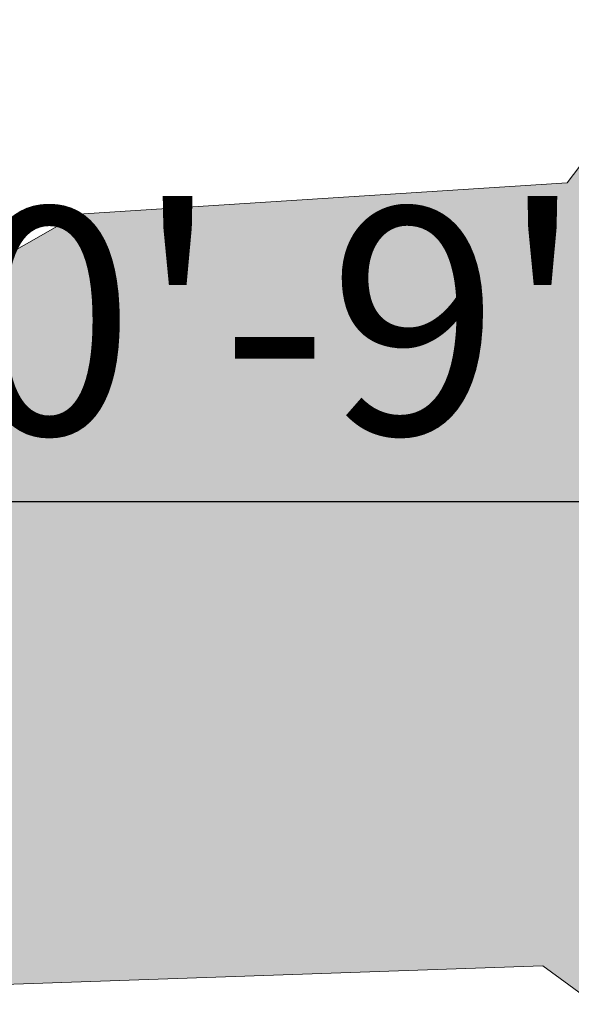
# Model space of a CAD drawing. Units: inches. Extents: x 2091 to 2899, y 967 to 2217.
# Tile 252 of 256: x 2221.88 to 2231.62, y 1131.25 to 1148.63. Entities that reach past the tile are written whole.
import ezdxf

# ---------------------------------------------------------------- set-up
doc = ezdxf.new("R2010")
doc.units = ezdxf.units.IN
doc.layers.add('A-ANNO-DIMS', color=2, linetype='Continuous', lineweight=18)
doc.layers.add('L-PLNT-TREE', color=94, linetype='Continuous', lineweight=13)
doc.layers.add('A-WALL-PATT', color=141, linetype='Continuous', lineweight=13, true_color=0xadddf7)
doc.layers.add('L-PLNT-PATT', color=114, linetype='Continuous', lineweight=13, true_color=0x139b48)
doc.styles.get("Standard").update_dxf_attribs({"font": 'arial.ttf'})
doc.dimstyles.new('ISO-25', dxfattribs={"dimtxt": 4, "dimasz": 4, "dimexe": 1.25, "dimexo": 0.625, "dimtad": 1, "dimdec": 0, "dimlunit": 3, "dimtxsty": 'Standard', "dimcen": 2.5, "dimadec": 0, "dimazin": 0, "dimtfac": 1, "dimtdec": 0, "dimtmove": 0, "dimatfit": 3, "dimfxl": 1, "dimarcsym": 0})

# ---------------------------------------------------------------- blocks, each defined once
blk = doc.blocks.new('*U25')
blk.add_lwpolyline([(-1139.42368, 1783.79628), (-1216.11644, 1685.47796), (-1117.5111, 1601.2033), (-1051.7759, 1643.3419), (-1126.09884, 1521.20092), (-1072.10606, 1527.49758), (-1079.90386, 1416.93646), (-1259.93906, 1179.83508), (-1479.05978, 1165.78888), (-1577.66258, 1109.60662), (-1742.00312, 927.01364), (-1676.26538, 814.64658), (-1270.89408, 828.69278), (-1194.20386, 772.51052), (-1007.95074, 856.78518), (-876.4778, 575.87134), (-821.70016, 575.87134), (-569.71184, 884.87504)])
blk = doc.blocks.new('*D37')
at = {"layer": 'A-ANNO-DIMS', "color": 0, "lineweight": -2, "transparency": 16777216}
for p, q in [((2203.116, 1151.622), (2203.116, 1138.874)), ((2212.276, 1151.622), (2212.276, 1138.874)), ((2199.116, 1140.124), (2195.116, 1140.124)), ((2203.116, 1140.124), (2212.276, 1140.124)), ((2216.276, 1140.124), (2245.908, 1140.124))]:
    blk.add_line(p, q, dxfattribs=at)
at = {"layer": 'A-ANNO-DIMS', "color": 0, "transparency": 16777216}
for points in [[(2199.116, 1140.79), (2199.116, 1139.457), (2203.116, 1140.124)], [(2216.276, 1140.79), (2216.276, 1139.457), (2212.276, 1140.124)]]:
    blk.add_solid(points, dxfattribs=at)
at = {"layer": 'Defpoints', "color": 0, "transparency": 16777216}
for p in [(2203.116, 1152.247), (2212.276, 1152.247), (2212.276, 1140.124)]:
    blk.add_point(p, dxfattribs=at)
at = {"layer": 'A-ANNO-DIMS', "color": 0, "transparency": 16777216, "insert": (2233.092, 1142.791), "char_height": 4, "attachment_point": 5}
blk.add_mtext('0\'-9" TYP.', dxfattribs=at)
blk = doc.blocks.new('*D71')
at = {"layer": 'A-ANNO-DIMS', "color": 0, "lineweight": -2, "transparency": 16777216}
for p, q in [((2212.144, 1351.294), (2212.144, 969.464)), ((2452.144, 1351.294), (2452.144, 969.464)), ((2216.144, 970.714), (2448.144, 970.714))]:
    blk.add_line(p, q, dxfattribs=at)
at = {"layer": 'A-ANNO-DIMS', "color": 0, "transparency": 16777216}
for points in [[(2216.144, 971.381), (2216.144, 970.048), (2212.144, 970.714)], [(2448.144, 971.381), (2448.144, 970.048), (2452.144, 970.714)]]:
    blk.add_solid(points, dxfattribs=at)
at = {"layer": 'Defpoints', "color": 0, "transparency": 16777216}
for p in [(2212.144, 1351.919), (2452.144, 1351.919), (2452.144, 970.714)]:
    blk.add_point(p, dxfattribs=at)
at = {"layer": 'A-ANNO-DIMS', "color": 0, "transparency": 16777216, "insert": (2332.144, 973.382), "char_height": 4, "attachment_point": 5}
blk.add_mtext('20\'-0"', dxfattribs=at)

msp = doc.modelspace()

# ---------------------------------------------------------------- hatches: boundary and pattern name
at = {"layer": 'A-WALL-PATT'}
h = msp.add_hatch(color=256, dxfattribs=at)
h.dxf.hatch_style = 1
h.paths.add_polyline_path([(2803.144, 2050.919), (2203.144, 2050.919), (2203.144, 1090.919), (2803.144, 1090.919)])
h.paths.add_polyline_path([(2635.799, 1147.54), (2674.524, 1147.54, 0.376086), (2678.53, 1152.88), (2678.53, 1159.556, 0.333335), (2674.524, 1163.562), (2674.524, 1163.562), (2674.524, 1192.934), (2635.806, 1192.934), (2597.088, 1192.934), (2597.088, 1163.562, 0.333335), (2593.082, 1159.556), (2593.082, 1152.88, 0.376086), (2597.088, 1147.54)], flags=0)
h.paths.add_polyline_path([(2436.01, 1278.241, 0.000483), (2435.953, 1278.215, -0.001328), (2435.936, 1278.112, -0.001711), (2436.116, 1278.041, 0.002185)], flags=0)
h.paths.add_polyline_path([(2794.144, 1143.419), (2794.144, 1347.419), (2543.37, 1347.419), (2543.37, 1351.919), (2794.144, 1351.919), (2794.144, 1392.714), (2793.947, 1392.714), (2793.947, 1473.537), (2794.144, 1473.537), (2794.144, 1531.919), (2650.144, 1531.919), (2650.144, 1536.419), (2794.144, 1536.419), (2794.144, 1692.419), (2609.376, 1692.419), (2609.376, 1644.419), (2604.876, 1644.419), (2604.876, 1744.919), (2609.376, 1744.919), (2609.376, 1696.919), (2794.144, 1696.919), (2794.144, 1780.919), (2609.644, 1780.919), (2493.876, 1780.919), (2493.876, 1785.419), (2609.644, 1785.419), (2794.144, 1785.419), (2794.144, 1847.939), (2793.951, 1847.939), (2793.951, 1928.762), (2794.144, 1928.762), (2794.144, 1941.419), (2614.144, 1941.419), (2614.144, 1821.419), (2609.644, 1821.419), (2609.644, 1941.419), (2392.144, 1941.419), (2392.144, 1819.919), (2387.644, 1819.919), (2387.644, 1941.419), (2212.144, 1941.419), (2212.144, 1783.919), (2392.144, 1783.919), (2392.144, 1780.919), (2212.144, 1780.919), (2212.144, 1629.419), (2387.644, 1629.419), (2387.644, 1744.919), (2392.144, 1744.919), (2392.144, 1627.919), (2317.144, 1627.919), (2317.144, 1551.419), (2317.144, 1536.419), (2459.384, 1536.419), (2459.384, 1602.396), (2463.884, 1602.396), (2463.884, 1531.919), (2456.644, 1531.919), (2456.644, 1529.919), (2452.144, 1529.919), (2452.144, 1531.919), (2312.644, 1531.919), (2312.644, 1551.419), (2306.144, 1551.419), (2306.144, 1555.919), (2308.144, 1555.919), (2308.144, 1551.419), (2312.644, 1551.419), (2312.644, 1627.919), (2212.144, 1627.919), (2212.144, 1555.919), (2270.144, 1555.919), (2270.144, 1551.419), (2212.144, 1551.419), (2212.144, 1351.919), (2272.144, 1351.919), (2272.144, 1347.419), (2212.144, 1347.419), (2212.144, 1275.419), (2308.144, 1275.419), (2308.144, 1351.919), (2452.144, 1351.919), (2452.144, 1493.919), (2456.644, 1493.919), (2456.644, 1347.419), (2312.644, 1347.419), (2312.644, 1270.919), (2212.144, 1270.919), (2212.144, 1099.919), (2281.238, 1099.919), (2282.871, 1110.914), (2282.008, 1116.997), (2278.558, 1121.42), (2268.206, 1128.056), (2272.088, 1128.056), (2273.813, 1131.927), (2279.42, 1134.692), (2285.028, 1135.245), (2287.616, 1137.457), (2288.047, 1138.01), (2289.341, 1140.775), (2291.067, 1139.669), (2292.361, 1135.245), (2295.38, 1136.904), (2296.243, 1135.798), (2297.105, 1133.033), (2300.125, 1138.01), (2303.144, 1138.01), (2304.438, 1135.798), (2303.144, 1133.586), (2306.595, 1134.692), (2307.889, 1133.033), (2310.908, 1135.245), (2313.927, 1134.139), (2315.627, 1132.427), (2308.32, 1117.55), (2290.204, 1109.808), (2288.91, 1103.172), (2289.272, 1099.919), (2434.918, 1099.919), (2431.593, 1124.788), (2429.93, 1169.553), (2430.927, 1240.52), (2435.659, 1238.186), (2437.135, 1196.554), (2438.798, 1143.973), (2442.678, 1111.998), (2446.558, 1099.919), (2794.144, 1099.919), (2794.144, 1138.919), (2548.032, 1138.919), (2548.032, 1143.419), (2548.032, 1148.819), (2546.668, 1148.032), (2528.686, 1179.179, 0.256256), (2512.032, 1148.819), (2512.032, 1143.419), (2512.032, 1138.919), (2507.532, 1138.919), (2507.532, 1143.419), (2507.532, 1148.819, 0.256256), (2490.879, 1179.179), (2472.896, 1148.032), (2471.532, 1148.819), (2471.532, 1143.419), (2467.032, 1143.419), (2467.032, 1269.946, 0.039061), (2460.91, 1273.58), (2467.032, 1273.58), (2467.032, 1286.325, 0.014511), (2465.216, 1286.762), (2467.032, 1287.053), (2467.032, 1323.419), (2471.532, 1323.419), (2471.532, 1148.819), (2489.532, 1179.996), (2490.896, 1179.208), (2490.879, 1179.179, -0.256256), (2507.532, 1148.819), (2507.532, 1143.419), (2512.032, 1143.419), (2512.032, 1148.819, -0.256256), (2528.686, 1179.179), (2528.668, 1179.208), (2530.032, 1179.996), (2548.032, 1148.819), (2548.032, 1143.419)], flags=16)
h.paths.add_polyline_path([(2607.769, 1200.945), (2607.769, 1265.031), (2597.088, 1281.052), (2619.785, 1281.052), (2627.795, 1337.127), (2635.799, 1337.127), (2643.817, 1337.127), (2651.827, 1281.052), (2674.524, 1281.052), (2663.843, 1265.031), (2663.843, 1200.945), (2635.806, 1200.945)], flags=0)
edge = h.paths.add_edge_path(flags=0)
edge.add_ellipse((13303.896, 1272.999), major_axis=(-10595.313, 0), ratio=0.84230387, start_angle=0.6282372, end_angle=0.6465541, ccw=False)
edge.add_ellipse((2711.7, 1156.853), major_axis=(2.22, 0), ratio=0.842304, start_angle=111.5352, end_angle=180.6282, ccw=False)
edge.add_ellipse((13303.156, 1272.999), major_axis=(-10593.026, 0), ratio=0.84230387, start_angle=0.5282715, end_angle=0.6465541, ccw=False)
edge.add_line((2710.765, 1175.333), (2710.13, 1175.333))
edge.add_ellipse((2710.13, 1176.58), major_axis=(1.48, 0), ratio=0.842304, start_angle=180, end_angle=270, ccw=False)
edge.add_line((2708.65, 1176.58), (2708.65, 1200.783))
edge.add_ellipse((2710.13, 1200.783), major_axis=(1.48, 0), ratio=0.842304, start_angle=90, end_angle=180, ccw=False)
edge.add_line((2710.13, 1202.029), (2710.465, 1202.029))
edge.add_ellipse((13303.156, 1272.999), major_axis=(-10593.026, 0), ratio=0.84230387, start_angle=-0.0902291, end_angle=0.3838668, ccw=False)
edge.add_ellipse((2710.13, 1290.927), major_axis=(-1.48, 0), ratio=0.842304, start_angle=0, end_angle=90, ccw=False)
edge.add_line((2708.65, 1290.927), (2708.65, 1315.13))
edge.add_ellipse((2710.13, 1315.13), major_axis=(-1.48, 0), ratio=0.842304, start_angle=-90, end_angle=0, ccw=False)
edge.add_line((2710.13, 1316.377), (2710.706, 1316.377))
edge.add_ellipse((3238.402, 1296.29), major_axis=(528.234, 0), ratio=0.8423039, start_angle=176.34957, end_angle=177.82005, ccw=False)
edge.add_ellipse((2775.063, 1071.451), major_axis=(313.308, 0), ratio=0.8423039, start_angle=102.12597, end_angle=103.78053, ccw=False)
edge.add_ellipse((2775.063, 1078.306), major_axis=(-305.303, 0), ratio=0.8423039, start_angle=-79.79046, end_angle=-77.55537, ccw=False)
edge.add_ellipse((2695.142, 1541.975), major_axis=(-250.96, 0), ratio=0.8423039, start_angle=99.25657, end_angle=102.55493)
edge.add_line((2741.41, 1334.214), (2747.133, 1337.378))
edge.add_ellipse((2747.539, 1336.857), major_axis=(-0.74, 0), ratio=0.842304, start_angle=270, end_angle=307.9331, ccw=False)
edge.add_ellipse((2747.539, 1336.857), major_axis=(-0.74, 0), ratio=0.842304, start_angle=232.0669, end_angle=270, ccw=False)
edge.add_line((2747.945, 1337.378), (2753.667, 1334.214))
edge.add_ellipse((2799.935, 1541.975), major_axis=(250.96, 0), ratio=0.8423039, start_angle=257.44507, end_angle=260.74343)
edge.add_ellipse((2720.014, 1078.306), major_axis=(305.303, 0), ratio=0.8423039, start_angle=77.55537, end_angle=79.79046, ccw=False)
edge.add_ellipse((2720.014, 1071.451), major_axis=(-313.308, 0), ratio=0.8423039, start_angle=256.21947, end_angle=257.87403, ccw=False)
edge.add_ellipse((2256.676, 1296.29), major_axis=(-528.234, 0), ratio=0.8423039, start_angle=182.17995, end_angle=183.65043, ccw=False)
edge.add_line((2784.371, 1316.377), (2784.947, 1316.377))
edge.add_ellipse((2784.947, 1315.13), major_axis=(1.48, 0), ratio=0.842304, start_angle=0, end_angle=90, ccw=False)
edge.add_line((2786.427, 1315.13), (2786.427, 1290.927))
edge.add_ellipse((2784.947, 1290.927), major_axis=(1.48, 0), ratio=0.842304, start_angle=270, end_angle=360, ccw=False)
edge.add_ellipse((-7808.079, 1272.999), major_axis=(10593.026, 0), ratio=0.84230387, start_angle=-0.3838668, end_angle=0.0902291, ccw=False)
edge.add_line((2784.612, 1202.029), (2784.947, 1202.029))
edge.add_ellipse((2784.947, 1200.783), major_axis=(1.48, 0), ratio=0.842304, start_angle=0, end_angle=90, ccw=False)
edge.add_line((2786.427, 1200.783), (2786.427, 1176.58))
edge.add_ellipse((2784.947, 1176.58), major_axis=(-1.48, 0), ratio=0.842304, start_angle=90, end_angle=180, ccw=False)
edge.add_line((2784.947, 1175.333), (2784.313, 1175.333))
edge.add_ellipse((-7808.079, 1272.999), major_axis=(10593.026, 0), ratio=0.84230387, start_angle=-0.6186432, end_angle=-0.5282715, ccw=False)
edge.add_ellipse((2783.377, 1156.853), major_axis=(-2.22, 0), ratio=0.842304, start_angle=179.3718, end_angle=248.4648, ccw=False)
edge.add_ellipse((-7808.819, 1272.999), major_axis=(-10595.313, 0), ratio=0.842303866, start_angle=179.3534459, end_angle=179.3717628, ccw=False)
edge.add_ellipse((2780.297, 1153.501), major_axis=(-5.246, 0), ratio=0.842304, start_angle=90, end_angle=179.3534, ccw=False)
edge.add_line((2780.297, 1149.082), (2714.78, 1149.082))
edge.add_ellipse((2714.78, 1153.501), major_axis=(5.246, 0), ratio=0.842304, start_angle=180.6466, end_angle=270, ccw=False)
edge = h.paths.add_edge_path(flags=0)
edge.add_line((2718.187, 1151.008), (2718.187, 1170.472))
edge.add_ellipse((2721.147, 1170.472), major_axis=(-2.96, 0), ratio=0.842304, start_angle=-90, end_angle=0, ccw=False)
edge.add_line((2721.147, 1172.965), (2773.93, 1172.965))
edge.add_ellipse((2773.93, 1170.472), major_axis=(-2.96, 0), ratio=0.842304, start_angle=180, end_angle=270, ccw=False)
edge.add_line((2776.89, 1170.472), (2776.89, 1151.008))
edge.add_line((2776.89, 1151.008), (2718.187, 1151.008))
edge = h.paths.add_edge_path(flags=0)
edge.add_line((2718.187, 1180.234), (2718.187, 1199.058))
edge.add_ellipse((2747.539, 1320.399), major_axis=(147.018, 0), ratio=0.8423039, start_angle=256.40187, end_angle=283.59813)
edge.add_line((2776.89, 1199.058), (2776.89, 1180.234))
edge.add_ellipse((2747.539, 1301.575), major_axis=(147.018, 0), ratio=0.8423039, start_angle=256.40187, end_angle=283.59813, ccw=False)
edge = h.paths.add_edge_path(flags=0)
edge.add_ellipse((13303.156, 1272.999), major_axis=(-10591.546, 0), ratio=0.84230387, start_angle=0.0555943, end_angle=0.3777642, ccw=False)
edge.add_line((2711.617, 1262.722), (2715.667, 1249.495))
edge.add_ellipse((6413.892, 1241.692), major_axis=(-3698.236, 0), ratio=0.84230387, start_angle=-0.120897, end_angle=0.364076)
edge.add_line((2715.761, 1218.192), (2711.934, 1203.167))
edge = h.paths.add_edge_path(flags=0)
edge.add_line((2718.187, 1251.075), (2716.002, 1267.45))
edge.add_ellipse((2742.151, 1202.19), major_axis=(81.773, 0), ratio=0.842304, start_angle=94.27742, end_angle=111.83495, ccw=False)
edge.add_line((2737.01, 1270.931), (2758.067, 1270.931))
edge.add_ellipse((2752.926, 1202.19), major_axis=(81.773, 0), ratio=0.842304, start_angle=68.16505, end_angle=85.72258, ccw=False)
edge.add_line((2779.075, 1267.45), (2776.89, 1251.075))
edge.add_ellipse((2750.338, 1187.885), major_axis=(79.58, 0), ratio=0.842304, start_angle=67.20809, end_angle=85.12993)
edge.add_line((2756.035, 1254.744), (2739.043, 1254.744))
edge.add_ellipse((2744.739, 1187.885), major_axis=(79.58, 0), ratio=0.842304, start_angle=94.87007, end_angle=112.79191)
edge = h.paths.add_edge_path(flags=0)
edge.add_line((2783.143, 1203.167), (2779.316, 1218.192))
edge.add_ellipse((-918.815, 1241.692), major_axis=(3698.236, 0), ratio=0.84230387, start_angle=-0.364076, end_angle=0.120897)
edge.add_line((2779.41, 1249.495), (2783.46, 1262.722))
edge.add_ellipse((-7808.079, 1272.999), major_axis=(-10591.546, 0), ratio=0.84230387, start_angle=179.6222358, end_angle=179.9444057, ccw=False)
edge = h.paths.add_edge_path(flags=0)
edge.add_ellipse((2734.201, 1286.69), major_axis=(-0.357, 6.34), ratio=0.603834, start_angle=89.002, end_angle=253.6574, ccw=False)
edge.add_line((2730.369, 1286.542), (2730.369, 1301.352))
edge.add_line((2730.369, 1301.352), (2735.913, 1305.215))
edge.add_ellipse((2736.385, 1304.735), major_axis=(0.74, 0), ratio=0.842304, start_angle=90, end_angle=134.4802, ccw=False)
edge.add_line((2736.385, 1305.358), (2738.033, 1305.358))
edge.add_line((2738.033, 1305.358), (2738.033, 1307.708))
edge.add_ellipse((2794.202, 1307.708), major_axis=(56.169, 0), ratio=0.842304, start_angle=150.5614, end_angle=180, ccw=False)
edge.add_ellipse((2700.876, 1307.708), major_axis=(-56.169, 0), ratio=0.842304, start_angle=180, end_angle=209.4386, ccw=False)
edge.add_line((2757.044, 1307.708), (2757.044, 1305.358))
edge.add_line((2757.044, 1305.358), (2758.692, 1305.358))
edge.add_ellipse((2758.692, 1304.735), major_axis=(-0.74, 0), ratio=0.842304, start_angle=225.5198, end_angle=270, ccw=False)
edge.add_line((2759.164, 1305.215), (2764.708, 1301.352))
edge.add_line((2764.708, 1301.352), (2764.708, 1286.542))
edge.add_ellipse((2760.876, 1286.69), major_axis=(0.357, 6.34), ratio=0.603834, start_angle=106.3426, end_angle=270.998, ccw=False)
edge.add_line((2757.044, 1285.797), (2757.044, 1307.708))
edge.add_ellipse((2700.876, 1307.708), major_axis=(-56.169, 0), ratio=0.842304, start_angle=180, end_angle=209.4386)
edge.add_ellipse((2794.202, 1307.708), major_axis=(56.169, 0), ratio=0.842304, start_angle=150.5614, end_angle=180)
edge.add_line((2738.033, 1307.708), (2738.033, 1285.797))
h.paths.add_polyline_path([(2417.812, 1104.45), (2413.492, 1102.53), (2410.612, 1103.97), (2409.172, 1106.37), (2407.252, 1107.33), (2406.292, 1109.73), (2405.332, 1114.05), (2405.332, 1117.89), (2406.292, 1120.13), (2407.252, 1119.81), (2408.848, 1118.328), (2410.174, 1119.424), (2410.211, 1120.406), (2411.041, 1121.419), (2410.699, 1119.859), (2410.174, 1119.424), (2410.088, 1117.176), (2411.133, 1116.206), (2413.972, 1119.33), (2416.852, 1120.77), (2416.87, 1120.799), (2417.035, 1119.405), (2417.896, 1118.143), (2418.292, 1118.37), (2419.544, 1120.039), (2419.361, 1118.387), (2419.032, 1119.356), (2418.399, 1118.512), (2419.252, 1114.53), (2418.794, 1107.199)], flags=0)
h.paths.add_polyline_path([(2508.87, 1347.419), (2508.37, 1347.419), (2508.37, 1351.919), (2508.87, 1351.919)], flags=0)
h.paths.add_polyline_path([(2473.37, 1347.419), (2472.37, 1347.419), (2467.87, 1347.419), (2467.87, 1455.419), (2472.37, 1455.419), (2472.37, 1352.419), (2473.37, 1352.419)], flags=0)
h.paths.add_polyline_path([(2352.106, 1217.446), (2349.226, 1218.886), (2347.786, 1221.286), (2345.866, 1222.246), (2344.906, 1224.646), (2343.946, 1228.966), (2343.946, 1232.806), (2344.906, 1235.046), (2345.866, 1234.726), (2347.462, 1233.244), (2348.788, 1234.341), (2348.825, 1235.322), (2349.655, 1236.336), (2349.313, 1234.775), (2348.788, 1234.341), (2348.702, 1232.093), (2349.747, 1231.123), (2352.586, 1234.246), (2355.466, 1235.686), (2355.484, 1235.715), (2355.649, 1234.322), (2356.51, 1233.06), (2356.906, 1233.286), (2358.158, 1234.956), (2357.975, 1233.304), (2357.646, 1234.273), (2357.013, 1233.428), (2357.866, 1229.446), (2357.408, 1222.115), (2356.426, 1219.366)], flags=0)
h.paths.add_polyline_path([(2348.297, 1112.224), (2347.014, 1112.31), (2345.53, 1114.127), (2345.732, 1115.858), (2346.812, 1116.982), (2346.812, 1114.646), (2345.867, 1114.214), (2346.88, 1114.3)], flags=0)
h.paths.add_polyline_path([(2347.014, 1110.926), (2346.272, 1110.493), (2346.61, 1111.186)], flags=0)
h.paths.add_polyline_path([(2345.867, 1118.194), (2345.53, 1117.329), (2343.708, 1118.021), (2344.383, 1118.626)], flags=0)
h.paths.add_polyline_path([(2346.677, 1109.282), (2346.07, 1108.071), (2345.867, 1110.061)], flags=0)
h.paths.add_polyline_path([(2345.057, 1119.751), (2343.64, 1119.751), (2343.978, 1121.135)], flags=0)
h.paths.add_polyline_path([(2345.26, 1116.55), (2345.125, 1115.858), (2344.922, 1115.685), (2344.72, 1116.377)], flags=0)
h.paths.add_polyline_path([(2345.665, 1112.31), (2345.462, 1111.532), (2344.045, 1111.964), (2344.652, 1112.57)], flags=0)
h.paths.add_polyline_path([(2345.192, 1113.349), (2344.45, 1113.868), (2344.72, 1114.387)], flags=0)
h.paths.add_polyline_path([(2344.652, 1116.809), (2344.18, 1115.685), (2344.652, 1115.339), (2343.91, 1114.906), (2343.033, 1115.944), (2343.64, 1116.463)], flags=0)
h.paths.add_polyline_path([(2345.867, 1106.686), (2344.99, 1105.562), (2344.517, 1106.6)], flags=0)
h.paths.add_polyline_path([(2344.855, 1110.061), (2344.517, 1109.282), (2344.113, 1109.715)], flags=0)
h.paths.add_polyline_path([(2344.045, 1113.522), (2343.438, 1113.089), (2342.763, 1113.954)], flags=0)
h.paths.add_polyline_path([(2344.315, 1111.012), (2342.965, 1110.32), (2342.965, 1111.099)], flags=0)
h.paths.add_polyline_path([(2345.125, 1104.697), (2344.585, 1103.745), (2344.45, 1104.264)], flags=0)
h.paths.add_polyline_path([(2342.83, 1121.222), (2341.75, 1120.53), (2340.536, 1121.049), (2340.131, 1121.828), (2340.671, 1122.952), (2341.143, 1121.828), (2341.615, 1122.001)], flags=0)
h.paths.add_polyline_path([(2342.965, 1119.751), (2343.033, 1118.453), (2342.088, 1118.021), (2342.02, 1119.491)], flags=0)
h.paths.add_polyline_path([(2342.695, 1116.896), (2341.953, 1116.636), (2342.02, 1117.329)], flags=0)
h.paths.add_polyline_path([(2343.033, 1112.224), (2342.02, 1111.791), (2341.548, 1112.224), (2342.358, 1113.349)], flags=0)
h.paths.add_polyline_path([(2343.775, 1104.437), (2342.628, 1102.88), (2342.695, 1104.61), (2343.438, 1105.129)], flags=0)
h.paths.add_polyline_path([(2342.02, 1115.079), (2340.806, 1115.512), (2340.941, 1116.377)], flags=0)
h.paths.add_polyline_path([(2341.481, 1120.097), (2341.481, 1119.405), (2341.076, 1119.578), (2341.143, 1120.097)], flags=0)
h.paths.add_polyline_path([(2341.818, 1114.473), (2340.941, 1113.089), (2340.806, 1114.56)], flags=0)
h.paths.add_polyline_path([(2341.143, 1118.54), (2340.941, 1116.982), (2339.051, 1117.675), (2339.051, 1118.626)], flags=0)
h.paths.add_polyline_path([(2342.695, 1101.668), (2341.953, 1101.841), (2342.56, 1102.361)], flags=0)
h.paths.add_polyline_path([(2340.333, 1119.665), (2338.444, 1119.578), (2337.904, 1120.357), (2339.658, 1120.616)], flags=0)
h.paths.add_polyline_path([(2340.333, 1115.339), (2340.063, 1113.695), (2339.388, 1115.339)], flags=0)
h.paths.add_polyline_path([(2341.818, 1103.831), (2341.548, 1102.88), (2341.143, 1103.658)], flags=0)
h.paths.add_polyline_path([(2339.051, 1122.866), (2337.296, 1121.828), (2337.094, 1123.125), (2337.769, 1123.818)], flags=0)
h.paths.add_polyline_path([(2339.118, 1121.741), (2338.848, 1121.222), (2338.174, 1121.049), (2338.376, 1121.568)], flags=0)
h.paths.add_polyline_path([(2339.186, 1119.319), (2338.646, 1118.713), (2338.241, 1118.107), (2338.241, 1118.886)], flags=0)
h.paths.add_polyline_path([(2341.143, 1101.928), (2340.603, 1101.236), (2340.063, 1101.841), (2340.603, 1102.361)], flags=0)
h.paths.add_polyline_path([(2337.634, 1117.761), (2336.621, 1118.28), (2337.296, 1118.972)], flags=0)
h.paths.add_polyline_path([(2336.824, 1119.578), (2334.799, 1118.972), (2335.204, 1120.357), (2336.554, 1120.876)], flags=0)
h.paths.add_polyline_path([(2339.118, 1100.457), (2337.364, 1100.543), (2336.756, 1101.236)], flags=0)
h.paths.add_polyline_path([(2336.351, 1122.433), (2336.014, 1121.914), (2334.934, 1122.433), (2334.529, 1123.471), (2335.744, 1122.779)], flags=0)
h.paths.add_polyline_path([(2334.732, 1120.876), (2334.259, 1120.357), (2334.057, 1120.789), (2334.597, 1121.308)], flags=0)
h.paths.add_polyline_path([(2334.462, 1122.174), (2332.572, 1121.308), (2331.357, 1122.174), (2332.1, 1122.866)], flags=0)
h.paths.add_polyline_path([(2334.259, 1118.54), (2333.382, 1118.453), (2333.652, 1119.319)], flags=0)
h.paths.add_polyline_path([(2335.542, 1102.274), (2334.192, 1102.62), (2335.272, 1103.312)], flags=0)
h.paths.add_polyline_path([(2332.707, 1119.665), (2331.695, 1120.443), (2332.505, 1120.789)], flags=0)
h.paths.add_polyline_path([(2334.732, 1101.149), (2333.517, 1101.582), (2333.989, 1101.755)], flags=0)
h.paths.add_polyline_path([(2332.64, 1116.636), (2331.087, 1116.29), (2331.965, 1118.194)], flags=0)
h.paths.add_polyline_path([(2330.75, 1121.568), (2330.277, 1120.27), (2328.523, 1119.319), (2328.995, 1121.049)], flags=0)
h.paths.add_polyline_path([(2330.75, 1118.626), (2330.008, 1117.502), (2329.873, 1118.021)], flags=0)
h.paths.add_polyline_path([(2332.1, 1102.361), (2330.547, 1102.014), (2331.695, 1102.966)], flags=0)
h.paths.add_polyline_path([(2329.535, 1113.608), (2329.063, 1112.31), (2328.59, 1113.349)], flags=0)
h.paths.add_polyline_path([(2328.388, 1117.848), (2327.51, 1116.55), (2327.173, 1117.761)], flags=0)
h.paths.add_polyline_path([(2329.738, 1106.513), (2329.535, 1105.302), (2328.253, 1106.081)], flags=0)
h.paths.add_polyline_path([(2328.658, 1114.387), (2328.05, 1114.127), (2328.32, 1114.906)], flags=0)
h.paths.add_polyline_path([(2328.32, 1112.224), (2327.106, 1112.137), (2326.701, 1112.656)], flags=0)
h.paths.add_polyline_path([(2326.903, 1115.252), (2326.701, 1114.127), (2325.216, 1113.608), (2326.093, 1115.339)], flags=0)
h.paths.add_polyline_path([(2326.633, 1108.33), (2326.093, 1107.379), (2325.891, 1108.503), (2326.498, 1109.109)], flags=0)
h.paths.add_polyline_path([(2615.144, 1531.919), (2609.644, 1531.919), (2609.644, 1620.419), (2614.144, 1620.419), (2614.144, 1536.419), (2615.144, 1536.419)], flags=0)
h.paths.add_polyline_path([(2545.144, 1563.419), (2464.144, 1563.419), (2464.144, 1632.419), (2509.144, 1632.419), (2509.144, 1627.919), (2509.144, 1603.919), (2468.644, 1603.919), (2468.644, 1567.919), (2540.644, 1567.919), (2540.644, 1591.919), (2545.144, 1591.919)], flags=0)
h.paths.add_polyline_path([(2388.969, 1549.986), (2357.434, 1549.986), (2357.434, 1623.361), (2399.363, 1623.361), (2435.689, 1623.361), (2435.593, 1602.559), (2435.593, 1602.396), (2388.969, 1602.396)], flags=0)
h.paths.add_polyline_path([(2388.881, 1555.809), (2374.904, 1555.809), (2374.904, 1600.572), (2374.904, 1615.458), (2406.351, 1615.458), (2406.351, 1618.939), (2412.174, 1615.458), (2406.351, 1611.976), (2406.351, 1615.458), (2388.881, 1615.458)], flags=0)
h.paths.add_polyline_path([(2568.876, 1644.419), (2453.376, 1644.419), (2453.376, 1785.419), (2457.876, 1785.419), (2457.876, 1648.919), (2568.876, 1648.919)], flags=0)
h.paths.add_polyline_path([(2212.144, 1945.919), (2212.144, 2041.919), (2794.144, 2041.919), (2794.144, 1945.919)], flags=16)
h.paths.add_polyline_path([(2271.083, 1964.317), (2776.853, 1964.317), (2776.853, 2037.17), (2271.083, 2037.17)], flags=8)
h.paths.add_polyline_path([(2380.649, 1536.824), (2461.041, 1536.824), (2461.041, 1554.653), (2380.649, 1554.653)], flags=8)
h.paths.add_polyline_path([(2240.756, 1609.725), (2309.186, 1609.725), (2309.186, 1617.698), (2240.756, 1617.698)], flags=8)
h.paths.add_polyline_path([(2212.677, 1313.504), (2282.592, 1313.504), (2282.592, 1322.745), (2212.677, 1322.745)], flags=8)
h.paths.add_polyline_path([(2457.112, 1114.779), (2558.482, 1114.779), (2558.482, 1142.22), (2457.112, 1142.22)], flags=8)
h.paths.add_polyline_path([(2473.442, 1273.01), (2604.641, 1273.01), (2604.641, 1318.347), (2473.442, 1318.347)], flags=8)
h.paths.add_polyline_path([(2638.876, 1626.977), (2684.25, 1627.977), (2684.038, 1637.597), (2638.664, 1636.598)], flags=8)
h.paths.add_polyline_path([(2537.591, 1453.793), (2628.39, 1453.793), (2628.39, 1475.345), (2537.591, 1475.345)], flags=8)
h.paths.add_polyline_path([(2504.138, 1714.632), (2554.647, 1714.632), (2554.647, 1730.238), (2504.138, 1730.238)], flags=8)
h.paths.add_polyline_path([(2487.501, 1575.652), (2535.097, 1575.652), (2535.097, 1598.378), (2487.501, 1598.378)], flags=8)
h.paths.add_polyline_path([(2709.099, 1735.71), (2740.017, 1735.71), (2740.017, 1749.938), (2709.099, 1749.938)], flags=8)
h.paths.add_polyline_path([(2442.438, 1792.172), (2564.729, 1792.172), (2564.729, 1842), (2442.438, 1842)], flags=8)
h.paths.add_polyline_path([(2655.816, 1809.644), (2789.52, 1806.694), (2790.085, 1832.292), (2656.381, 1835.242)], flags=8)
h.paths.add_polyline_path([(2234.843, 1797.72), (2368.593, 1794.769), (2369.161, 1820.504), (2235.411, 1823.455)], flags=8)
h.paths.add_polyline_path([(2245.138, 1644.006), (2398.428, 1640.624), (2398.995, 1666.325), (2245.706, 1669.707)], flags=8)
h.paths.add_polyline_path([(2306.143, 1431.169), (2413.768, 1428.794), (2414.333, 1454.392), (2306.708, 1456.766)], flags=8)
h.paths.add_polyline_path([(2306.835, 1458.233), (2393.38, 1456.323), (2393.933, 1481.354), (2307.387, 1483.264)], flags=8)
at = {"layer": 'L-PLNT-PATT'}
h = msp.add_hatch(color=256, dxfattribs=at)
h.dxf.hatch_style = 1
h.paths.add_polyline_path([(2333.338, 1165.659), (2329.024, 1166.212), (2331.612, 1168.424), (2335.063, 1177.271), (2328.162, 1184.46), (2319.535, 1187.225), (2323.417, 1193.308), (2319.966, 1203.814), (2317.809, 1203.814), (2313.496, 1213.215), (2310.908, 1212.662), (2307.889, 1212.662), (2305.732, 1217.086), (2307.026, 1223.168), (2310.477, 1223.168), (2304.007, 1230.91), (2303.136, 1237.046), (2299.693, 1240.864), (2296.674, 1237.546), (2294.949, 1238.652), (2294.517, 1241.417), (2292.361, 1242.523), (2289.341, 1239.758), (2285.89, 1240.311), (2283.302, 1235.334), (2283.302, 1230.91), (2286.753, 1229.251), (2284.165, 1227.592), (2281.577, 1229.804), (2274.244, 1222.615), (2274.244, 1220.957), (2271.225, 1219.298), (2272.088, 1217.639), (2274.244, 1214.321), (2270.362, 1211.556), (2266.48, 1214.321), (2264.324, 1213.768), (2263.461, 1211.556), (2266.48, 1211.003), (2266.912, 1206.579), (2263.539, 1207.132), (2259.579, 1203.261), (2263.892, 1202.708), (2262.167, 1197.178), (2258.285, 1196.625), (2253.971, 1193.861), (2248.795, 1191.096), (2248.364, 1193.308), (2244.482, 1185.013), (2251.383, 1186.672), (2255.697, 1183.907), (2254.403, 1177.271), (2246.639, 1174.506), (2243.188, 1176.718), (2241.894, 1173.4), (2238.875, 1172.847), (2236.287, 1169.53), (2233.267, 1165.659), (2237.149, 1162.341), (2239.737, 1164), (2236.811, 1159.191), (2238.937, 1159.439), (2238.63, 1155.086), (2231.542, 1145.752), (2222.915, 1145.199), (2219.033, 1142.987), (2212.563, 1135.798), (2215.151, 1131.374), (2231.111, 1131.927), (2234.13, 1129.715), (2241.463, 1133.033), (2246.639, 1121.973), (2248.795, 1121.973), (2258.716, 1134.139), (2261.736, 1135.798), (2263.892, 1133.033), (2263.892, 1129.162), (2267.343, 1128.056), (2272.088, 1128.056), (2273.813, 1131.927), (2279.42, 1134.692), (2285.028, 1135.245), (2287.616, 1137.457), (2288.047, 1138.01), (2289.341, 1140.775), (2291.067, 1139.669), (2292.361, 1135.245), (2295.38, 1136.904), (2296.243, 1135.798), (2297.105, 1133.033), (2300.125, 1138.01), (2303.144, 1138.01), (2304.438, 1135.798), (2303.144, 1133.586), (2306.595, 1134.692), (2307.889, 1133.033), (2310.908, 1135.245), (2313.927, 1134.139), (2319.966, 1128.056), (2322.554, 1126.95), (2324.711, 1124.738), (2342.827, 1126.397), (2346.278, 1123.079), (2348.866, 1124.185), (2341.964, 1133.033), (2341.533, 1136.351), (2343.69, 1139.669), (2339.808, 1150.175), (2337.651, 1150.175)])
h.paths.add_polyline_path([(2339.658, 1120.616), (2337.904, 1120.357), (2338.444, 1119.578), (2340.333, 1119.665)])
h.paths.add_polyline_path([(2341.143, 1118.54), (2339.051, 1118.626), (2339.051, 1117.675), (2340.941, 1116.982)])
h.paths.add_polyline_path([(2336.554, 1120.876), (2335.204, 1120.357), (2334.799, 1118.972), (2336.824, 1119.578)])
h.paths.add_polyline_path([(2337.296, 1118.972), (2336.621, 1118.28), (2337.634, 1117.761)])
h.paths.add_polyline_path([(2338.646, 1118.713), (2339.186, 1119.319), (2338.241, 1118.886), (2338.241, 1118.107)])
h.paths.add_polyline_path([(2339.051, 1122.866), (2337.769, 1123.818), (2337.094, 1123.125), (2337.296, 1121.828)])
h.paths.add_polyline_path([(2341.615, 1122.001), (2341.143, 1121.828), (2340.671, 1122.952), (2340.131, 1121.828), (2340.536, 1121.049), (2341.75, 1120.53), (2342.83, 1121.222)])
h.paths.add_polyline_path([(2342.965, 1119.751), (2342.02, 1119.491), (2342.088, 1118.021), (2343.033, 1118.453)])
h.paths.add_polyline_path([(2345.867, 1118.194), (2344.383, 1118.626), (2343.708, 1118.021), (2345.53, 1117.329)])
h.paths.add_polyline_path([(2344.652, 1116.809), (2343.64, 1116.463), (2343.033, 1115.944), (2343.91, 1114.906), (2344.652, 1115.339), (2344.18, 1115.685)])
h.paths.add_polyline_path([(2346.812, 1116.982), (2345.732, 1115.858), (2345.53, 1114.127), (2347.014, 1112.31), (2348.297, 1112.224), (2346.88, 1114.3), (2345.867, 1114.214), (2346.812, 1114.646)])
h.paths.add_polyline_path([(2345.26, 1116.55), (2344.72, 1116.377), (2344.922, 1115.685), (2345.125, 1115.858)])
h.paths.add_polyline_path([(2342.695, 1116.896), (2342.02, 1117.329), (2341.953, 1116.636)])
h.paths.add_polyline_path([(2341.481, 1120.097), (2341.143, 1120.097), (2341.076, 1119.578), (2341.481, 1119.405)])
h.paths.add_polyline_path([(2343.978, 1121.135), (2343.64, 1119.751), (2345.057, 1119.751)])
h.paths.add_polyline_path([(2339.118, 1121.741), (2338.376, 1121.568), (2338.174, 1121.049), (2338.848, 1121.222)])
h.paths.add_polyline_path([(2336.351, 1122.433), (2335.744, 1122.779), (2334.529, 1123.471), (2334.934, 1122.433), (2336.014, 1121.914)])
h.paths.add_polyline_path([(2334.462, 1122.174), (2332.1, 1122.866), (2331.357, 1122.174), (2332.572, 1121.308)])
h.paths.add_polyline_path([(2334.597, 1121.308), (2334.057, 1120.789), (2334.259, 1120.357), (2334.732, 1120.876)])
h.paths.add_polyline_path([(2332.505, 1120.789), (2331.695, 1120.443), (2332.707, 1119.665)])
h.paths.add_polyline_path([(2333.652, 1119.319), (2333.382, 1118.453), (2334.259, 1118.54)])
h.paths.add_polyline_path([(2331.965, 1118.194), (2331.087, 1116.29), (2332.64, 1116.636)])
h.paths.add_polyline_path([(2330.75, 1121.568), (2328.995, 1121.049), (2328.523, 1119.319), (2330.277, 1120.27)])
h.paths.add_polyline_path([(2330.75, 1118.626), (2329.873, 1118.021), (2330.008, 1117.502)])
h.paths.add_polyline_path([(2328.388, 1117.848), (2327.173, 1117.761), (2327.51, 1116.55)])
h.paths.add_polyline_path([(2326.903, 1115.252), (2326.093, 1115.339), (2325.216, 1113.608), (2326.701, 1114.127)])
h.paths.add_polyline_path([(2328.658, 1114.387), (2328.32, 1114.906), (2328.05, 1114.127)])
h.paths.add_polyline_path([(2326.701, 1112.656), (2327.106, 1112.137), (2328.32, 1112.224)])
h.paths.add_polyline_path([(2329.535, 1113.608), (2328.59, 1113.349), (2329.063, 1112.31)])
h.paths.add_polyline_path([(2340.333, 1115.339), (2339.388, 1115.339), (2340.063, 1113.695)])
h.paths.add_polyline_path([(2340.941, 1116.377), (2340.806, 1115.512), (2342.02, 1115.079)])
h.paths.add_polyline_path([(2341.818, 1114.473), (2340.806, 1114.56), (2340.941, 1113.089)])
h.paths.add_polyline_path([(2343.033, 1112.224), (2342.358, 1113.349), (2341.548, 1112.224), (2342.02, 1111.791)])
h.paths.add_polyline_path([(2342.763, 1113.954), (2343.438, 1113.089), (2344.045, 1113.522)])
h.paths.add_polyline_path([(2344.72, 1114.387), (2344.45, 1113.868), (2345.192, 1113.349)])
h.paths.add_polyline_path([(2345.665, 1112.31), (2344.652, 1112.57), (2344.045, 1111.964), (2345.462, 1111.532)])
h.paths.add_polyline_path([(2344.315, 1111.012), (2342.965, 1111.099), (2342.965, 1110.32)])
h.paths.add_polyline_path([(2344.855, 1110.061), (2344.113, 1109.715), (2344.517, 1109.282)])
h.paths.add_polyline_path([(2346.677, 1109.282), (2345.867, 1110.061), (2346.07, 1108.071)])
h.paths.add_polyline_path([(2347.014, 1110.926), (2346.61, 1111.186), (2346.272, 1110.493)])
h.paths.add_polyline_path([(2345.867, 1106.686), (2344.517, 1106.6), (2344.99, 1105.562)])
h.paths.add_polyline_path([(2345.125, 1104.697), (2344.45, 1104.264), (2344.585, 1103.745)])
h.paths.add_polyline_path([(2343.775, 1104.437), (2343.438, 1105.129), (2342.695, 1104.61), (2342.628, 1102.88)])
h.paths.add_polyline_path([(2341.818, 1103.831), (2341.143, 1103.658), (2341.548, 1102.88)])
h.paths.add_polyline_path([(2342.56, 1102.361), (2341.953, 1101.841), (2342.695, 1101.668)])
h.paths.add_polyline_path([(2341.143, 1101.928), (2340.603, 1102.361), (2340.063, 1101.841), (2340.603, 1101.236)])
h.paths.add_polyline_path([(2336.756, 1101.236), (2337.364, 1100.543), (2339.118, 1100.457)])
h.paths.add_polyline_path([(2335.272, 1103.312), (2334.192, 1102.62), (2335.542, 1102.274)])
h.paths.add_polyline_path([(2333.989, 1101.755), (2333.517, 1101.582), (2334.732, 1101.149)])
h.paths.add_polyline_path([(2331.695, 1102.966), (2330.547, 1102.014), (2332.1, 1102.361)])
h.paths.add_polyline_path([(2329.738, 1106.513), (2328.253, 1106.081), (2329.535, 1105.302)])
h.paths.add_polyline_path([(2326.633, 1108.33), (2326.498, 1109.109), (2325.891, 1108.503), (2326.093, 1107.379)])
h.paths.add_polyline_path([(2240.596, 1257.814), (2239.584, 1257.468), (2238.977, 1256.949), (2239.854, 1255.911), (2240.596, 1256.344), (2240.124, 1256.69)])
h.paths.add_polyline_path([(2241.811, 1259.199), (2240.327, 1259.631), (2239.652, 1259.026), (2241.474, 1258.334)])
h.paths.add_polyline_path([(2242.756, 1257.987), (2241.676, 1256.863), (2241.474, 1255.132), (2242.958, 1253.315), (2244.241, 1253.229), (2242.824, 1255.305), (2241.811, 1255.219), (2242.756, 1255.651)])
h.paths.add_polyline_path([(2241.609, 1253.315), (2240.596, 1253.575), (2239.989, 1252.969), (2241.406, 1252.537)])
h.paths.add_polyline_path([(2240.664, 1255.392), (2240.394, 1254.873), (2241.136, 1254.354)])
h.paths.add_polyline_path([(2242.958, 1251.931), (2242.554, 1252.191), (2242.216, 1251.498)])
h.paths.add_polyline_path([(2240.259, 1252.017), (2238.909, 1252.104), (2238.909, 1251.325)])
h.paths.add_polyline_path([(2238.302, 1254.354), (2237.492, 1253.229), (2237.964, 1252.796), (2238.977, 1253.229)])
h.paths.add_polyline_path([(2239.989, 1254.527), (2238.707, 1254.959), (2239.382, 1254.094)])
h.paths.add_polyline_path([(2240.799, 1251.066), (2240.057, 1250.72), (2240.461, 1250.287)])
h.paths.add_polyline_path([(2241.811, 1251.066), (2242.014, 1249.076), (2242.621, 1250.287)])
h.paths.add_polyline_path([(2241.204, 1257.555), (2240.664, 1257.382), (2240.866, 1256.69), (2241.069, 1256.863)])
h.paths.add_polyline_path([(2238.639, 1257.901), (2237.964, 1258.334), (2237.897, 1257.641)])
h.paths.add_polyline_path([(2238.909, 1260.756), (2237.964, 1260.496), (2238.032, 1259.026), (2238.977, 1259.458)])
h.paths.add_polyline_path([(2239.922, 1262.14), (2239.584, 1260.756), (2241.001, 1260.756)])
h.paths.add_polyline_path([(2238.774, 1262.227), (2237.559, 1263.006), (2237.087, 1262.833), (2236.615, 1263.957), (2236.075, 1262.833), (2236.48, 1262.054), (2237.694, 1261.535)])
h.paths.add_polyline_path([(2237.425, 1261.102), (2237.087, 1261.102), (2237.02, 1260.583), (2237.425, 1260.41)])
h.paths.add_polyline_path([(2237.087, 1259.545), (2234.995, 1259.631), (2234.995, 1258.68), (2236.885, 1257.987)])
h.paths.add_polyline_path([(2236.885, 1257.382), (2236.75, 1256.517), (2237.964, 1256.084)])
h.paths.add_polyline_path([(2237.762, 1255.478), (2236.75, 1255.565), (2236.885, 1254.094)])
h.paths.add_polyline_path([(2236.277, 1256.344), (2235.332, 1256.344), (2236.007, 1254.7)])
h.paths.add_polyline_path([(2241.811, 1247.691), (2240.461, 1247.605), (2240.934, 1246.567)])
h.paths.add_polyline_path([(2239.719, 1245.442), (2239.382, 1246.134), (2238.639, 1245.615), (2238.572, 1243.885)])
h.paths.add_polyline_path([(2241.069, 1245.702), (2240.394, 1245.269), (2240.529, 1244.75)])
h.paths.add_polyline_path([(2237.762, 1244.836), (2237.087, 1244.663), (2237.492, 1243.885)])
h.paths.add_polyline_path([(2237.087, 1242.933), (2236.547, 1243.366), (2236.007, 1242.846), (2236.547, 1242.241)])
h.paths.add_polyline_path([(2238.504, 1243.366), (2237.897, 1242.846), (2238.639, 1242.673)])
h.paths.add_polyline_path([(2232.7, 1242.241), (2233.308, 1241.548), (2235.062, 1241.462)], flags=17)
h.paths.add_polyline_path([(2231.216, 1244.317), (2230.136, 1243.625), (2231.486, 1243.279)])
h.paths.add_polyline_path([(2229.933, 1242.76), (2229.461, 1242.587), (2230.676, 1242.154)])
h.paths.add_polyline_path([(2227.639, 1243.971), (2226.491, 1243.019), (2228.044, 1243.366)])
h.paths.add_polyline_path([(2222.577, 1249.335), (2222.442, 1250.114), (2221.835, 1249.508), (2222.037, 1248.384)])
h.paths.add_polyline_path([(2225.682, 1247.518), (2224.197, 1247.086), (2225.479, 1246.307)])
h.paths.add_polyline_path([(2225.479, 1254.613), (2224.534, 1254.354), (2225.007, 1253.315)])
h.paths.add_polyline_path([(2224.264, 1253.229), (2222.645, 1253.661), (2223.05, 1253.142)])
h.paths.add_polyline_path([(2222.847, 1256.257), (2222.037, 1256.344), (2221.16, 1254.613), (2222.645, 1255.132)])
h.paths.add_polyline_path([(2224.332, 1258.853), (2223.117, 1258.766), (2223.454, 1257.555)])
h.paths.add_polyline_path([(2226.694, 1259.631), (2225.817, 1259.026), (2225.952, 1258.507)])
h.paths.add_polyline_path([(2227.909, 1259.199), (2227.031, 1257.295), (2228.584, 1257.641)])
h.paths.add_polyline_path([(2224.264, 1255.911), (2223.994, 1255.132), (2224.602, 1255.392)])
h.paths.add_polyline_path([(2229.596, 1260.324), (2229.326, 1259.458), (2230.203, 1259.545)])
h.paths.add_polyline_path([(2228.449, 1261.794), (2227.639, 1261.448), (2228.651, 1260.67)])
h.paths.add_polyline_path([(2230.406, 1263.179), (2228.044, 1263.871), (2227.301, 1263.179), (2228.516, 1262.313)])
h.paths.add_polyline_path([(2232.768, 1260.583), (2232.498, 1261.881), (2231.148, 1261.362), (2230.743, 1259.977)])
h.paths.add_polyline_path([(2230.676, 1261.881), (2230.541, 1262.313), (2230.001, 1261.794), (2230.203, 1261.362)])
h.paths.add_polyline_path([(2232.295, 1263.438), (2231.688, 1263.784), (2230.473, 1264.476), (2230.878, 1263.438), (2231.958, 1262.919)])
h.paths.add_polyline_path([(2234.995, 1263.871), (2233.713, 1264.823), (2233.038, 1264.13), (2233.24, 1262.833)])
h.paths.add_polyline_path([(2235.062, 1262.746), (2234.32, 1262.573), (2234.118, 1262.054), (2234.792, 1262.227)])
h.paths.add_polyline_path([(2235.602, 1261.621), (2233.848, 1261.362), (2234.388, 1260.583), (2236.277, 1260.67)])
h.paths.add_polyline_path([(2235.13, 1260.324), (2234.185, 1259.891), (2234.185, 1259.112), (2234.59, 1259.718)])
h.paths.add_polyline_path([(2226.694, 1262.573), (2224.939, 1262.054), (2224.467, 1260.324), (2226.221, 1261.275)])
h.paths.add_polyline_path([(2233.24, 1259.977), (2232.565, 1259.285), (2233.578, 1258.766)])
h.paths.add_polyline_path([(2337.267, 1337.827), (2336.187, 1336.703), (2335.985, 1334.972), (2337.469, 1333.155), (2338.752, 1333.069), (2337.335, 1335.145), (2336.322, 1335.059), (2337.267, 1335.491)])
h.paths.add_polyline_path([(2336.322, 1339.039), (2334.838, 1339.471), (2334.163, 1338.866), (2335.985, 1338.174)])
h.paths.add_polyline_path([(2334.433, 1341.98), (2334.095, 1340.596), (2335.512, 1340.596)])
h.paths.add_polyline_path([(2333.285, 1342.067), (2332.07, 1342.846), (2331.598, 1342.673), (2331.126, 1343.797), (2330.586, 1342.673), (2330.991, 1341.894), (2332.205, 1341.375)])
h.paths.add_polyline_path([(2333.42, 1340.596), (2332.475, 1340.336), (2332.543, 1338.866), (2333.488, 1339.298)])
h.paths.add_polyline_path([(2331.936, 1340.942), (2331.598, 1340.942), (2331.531, 1340.423), (2331.936, 1340.25)])
h.paths.add_polyline_path([(2329.573, 1342.586), (2328.831, 1342.413), (2328.629, 1341.894), (2329.303, 1342.067)])
h.paths.add_polyline_path([(2329.506, 1343.711), (2328.224, 1344.663), (2327.549, 1343.97), (2327.751, 1342.673)])
h.paths.add_polyline_path([(2330.113, 1341.461), (2328.359, 1341.202), (2328.899, 1340.423), (2330.788, 1340.51)])
h.paths.add_polyline_path([(2331.598, 1339.385), (2329.506, 1339.471), (2329.506, 1338.52), (2331.396, 1337.827)])
h.paths.add_polyline_path([(2327.009, 1341.721), (2325.659, 1341.202), (2325.254, 1339.817), (2327.279, 1340.423)])
h.paths.add_polyline_path([(2326.806, 1343.278), (2326.199, 1343.624), (2324.984, 1344.316), (2325.389, 1343.278), (2326.469, 1342.759)])
h.paths.add_polyline_path([(2324.917, 1343.019), (2322.555, 1343.711), (2321.812, 1343.019), (2323.027, 1342.153)])
h.paths.add_polyline_path([(2321.205, 1342.413), (2319.45, 1341.894), (2318.978, 1340.164), (2320.732, 1341.115)])
h.paths.add_polyline_path([(2318.843, 1338.693), (2317.628, 1338.606), (2317.965, 1337.395)])
h.paths.add_polyline_path([(2322.42, 1339.039), (2321.542, 1337.135), (2323.095, 1337.481)])
h.paths.add_polyline_path([(2324.107, 1340.164), (2323.837, 1339.298), (2324.714, 1339.385)])
h.paths.add_polyline_path([(2322.96, 1341.634), (2322.15, 1341.288), (2323.162, 1340.51)])
h.paths.add_polyline_path([(2325.187, 1341.721), (2325.052, 1342.153), (2324.512, 1341.634), (2324.714, 1341.202)])
h.paths.add_polyline_path([(2321.205, 1339.471), (2320.328, 1338.866), (2320.463, 1338.347)])
h.paths.add_polyline_path([(2317.358, 1336.097), (2316.548, 1336.184), (2315.671, 1334.453), (2317.156, 1334.972)])
h.paths.add_polyline_path([(2318.775, 1335.751), (2318.505, 1334.972), (2319.113, 1335.232)])
h.paths.add_polyline_path([(2319.99, 1334.453), (2319.045, 1334.194), (2319.518, 1333.155)])
h.paths.add_polyline_path([(2317.156, 1333.501), (2317.561, 1332.982), (2318.775, 1333.069)])
h.paths.add_polyline_path([(2317.088, 1329.175), (2316.953, 1329.954), (2316.346, 1329.348), (2316.548, 1328.224)])
h.paths.add_polyline_path([(2320.193, 1327.358), (2318.708, 1326.926), (2319.99, 1326.147)])
h.paths.add_polyline_path([(2322.15, 1323.811), (2321.002, 1322.859), (2322.555, 1323.206)])
h.paths.add_polyline_path([(2325.727, 1324.157), (2324.647, 1323.465), (2325.997, 1323.119)])
h.paths.add_polyline_path([(2334.23, 1325.282), (2333.893, 1325.974), (2333.15, 1325.455), (2333.083, 1323.725)])
h.paths.add_polyline_path([(2336.322, 1327.531), (2334.972, 1327.445), (2335.445, 1326.407)])
h.paths.add_polyline_path([(2335.31, 1330.906), (2334.568, 1330.56), (2334.972, 1330.127)])
h.paths.add_polyline_path([(2334.77, 1331.857), (2333.42, 1331.944), (2333.42, 1331.165)])
h.paths.add_polyline_path([(2332.813, 1334.194), (2332.003, 1333.069), (2332.475, 1332.636), (2333.488, 1333.069)])
h.paths.add_polyline_path([(2335.107, 1333.415), (2334.5, 1332.809), (2335.917, 1332.377), (2336.12, 1333.155)])
h.paths.add_polyline_path([(2334.635, 1336.53), (2335.107, 1337.654), (2334.095, 1337.308), (2333.488, 1336.789), (2334.365, 1335.751), (2335.107, 1336.184)])
h.paths.add_polyline_path([(2335.715, 1337.395), (2335.175, 1337.222), (2335.377, 1336.53), (2335.58, 1336.703)])
h.paths.add_polyline_path([(2333.15, 1337.741), (2332.475, 1338.174), (2332.408, 1337.481)])
h.paths.add_polyline_path([(2330.788, 1336.184), (2329.843, 1336.184), (2330.518, 1334.54)])
h.paths.add_polyline_path([(2332.273, 1335.318), (2331.261, 1335.405), (2331.396, 1333.934)])
h.paths.add_polyline_path([(2331.396, 1337.222), (2331.261, 1336.357), (2332.475, 1335.924)])
h.paths.add_polyline_path([(2334.5, 1334.367), (2333.218, 1334.799), (2333.893, 1333.934)])
h.paths.add_polyline_path([(2335.175, 1335.232), (2334.905, 1334.713), (2335.647, 1334.194)])
h.paths.add_polyline_path([(2337.132, 1330.127), (2336.322, 1330.906), (2336.525, 1328.916)])
h.paths.add_polyline_path([(2337.065, 1332.031), (2336.727, 1331.338), (2337.469, 1331.771)])
h.paths.add_polyline_path([(2329.641, 1340.164), (2328.696, 1339.731), (2328.696, 1338.952), (2329.101, 1339.558)])
h.paths.add_polyline_path([(2327.751, 1339.817), (2327.076, 1339.125), (2328.089, 1338.606)])
h.paths.add_polyline_path([(2327.211, 1322.081), (2327.819, 1321.388), (2329.573, 1321.302)])
h.paths.add_polyline_path([(2324.444, 1322.6), (2323.972, 1322.427), (2325.187, 1321.994)])
h.paths.add_polyline_path([(2331.058, 1323.206), (2330.518, 1322.686), (2331.058, 1322.081), (2331.598, 1322.773)])
h.paths.add_polyline_path([(2332.273, 1324.676), (2331.598, 1324.503), (2332.003, 1323.725)])
h.paths.add_polyline_path([(2333.015, 1323.206), (2332.408, 1322.686), (2333.15, 1322.513)])
h.paths.add_polyline_path([(2335.58, 1325.542), (2334.905, 1325.109), (2335.04, 1324.59)])
h.paths.add_polyline_path([(2271.083, 1964.317), (2776.853, 1964.317), (2776.853, 2037.17), (2271.083, 2037.17)], flags=9)
h.paths.add_polyline_path([(2380.649, 1536.824), (2461.041, 1536.824), (2461.041, 1554.653), (2380.649, 1554.653)], flags=9)
h.paths.add_polyline_path([(2240.756, 1609.725), (2309.186, 1609.725), (2309.186, 1617.698), (2240.756, 1617.698)], flags=9)
h.paths.add_polyline_path([(2212.677, 1313.504), (2282.592, 1313.504), (2282.592, 1322.745), (2212.677, 1322.745)], flags=9)
h.paths.add_polyline_path([(2457.112, 1114.779), (2558.482, 1114.779), (2558.482, 1142.22), (2457.112, 1142.22)], flags=9)
h.paths.add_polyline_path([(2473.442, 1273.01), (2604.641, 1273.01), (2604.641, 1318.347), (2473.442, 1318.347)], flags=9)
h.paths.add_polyline_path([(2638.876, 1626.977), (2684.25, 1627.977), (2684.038, 1637.597), (2638.664, 1636.598)], flags=9)
h.paths.add_polyline_path([(2537.591, 1453.793), (2628.39, 1453.793), (2628.39, 1475.345), (2537.591, 1475.345)], flags=9)
h.paths.add_polyline_path([(2504.138, 1714.632), (2554.647, 1714.632), (2554.647, 1730.238), (2504.138, 1730.238)], flags=9)
h.paths.add_polyline_path([(2487.501, 1575.652), (2535.097, 1575.652), (2535.097, 1598.378), (2487.501, 1598.378)], flags=9)
h.paths.add_polyline_path([(2709.099, 1735.71), (2740.017, 1735.71), (2740.017, 1749.938), (2709.099, 1749.938)], flags=9)
h.paths.add_polyline_path([(2442.438, 1792.172), (2564.729, 1792.172), (2564.729, 1842), (2442.438, 1842)], flags=9)
h.paths.add_polyline_path([(2655.816, 1809.644), (2789.52, 1806.694), (2790.085, 1832.292), (2656.381, 1835.242)], flags=9)
h.paths.add_polyline_path([(2234.843, 1797.72), (2368.593, 1794.769), (2369.161, 1820.504), (2235.411, 1823.455)], flags=9)
h.paths.add_polyline_path([(2245.138, 1644.006), (2398.428, 1640.624), (2398.995, 1666.325), (2245.706, 1669.707)], flags=9)
h.paths.add_polyline_path([(2306.143, 1431.169), (2413.768, 1428.794), (2414.333, 1454.392), (2306.708, 1456.766)], flags=9)
h.paths.add_polyline_path([(2306.835, 1458.233), (2393.38, 1456.323), (2393.933, 1481.354), (2307.387, 1483.264)], flags=9)

# ---------------------------------------------------------------- block references
at = {"layer": 'L-PLNT-TREE', "xscale": 0.0393700787401575, "yscale": 0.0393700787401575, "zscale": 0.0393700787401575}
msp.add_blockref('*U25', (2281.146, 1099.301), dxfattribs=at)

# ---------------------------------------------------------------- dimensions: what is measured, and where the dimension line sits
at = {"layer": 'A-ANNO-DIMS'}
dim = msp.add_linear_dim(base=(2452.144, 970.714), p1=(2212.144, 1351.919), p2=(2452.144, 1351.919), dimstyle='ISO-25', override={"dimdec": 1, "dimlfac": 1, "dimrnd": 0, "dimzin": 1, "dimdsep": 46, "dimlunit": 4, "dimfrac": 2}, dxfattribs=at)
dim.commit()
dim.dimension.update_dxf_attribs({"geometry": '*D71', "text_midpoint": (2332.144, 973.382)})
dim = msp.add_linear_dim(base=(2212.276, 1140.124), p1=(2203.116, 1152.247), p2=(2212.276, 1152.247), text='<> TYP.', dimstyle='ISO-25', override={"dimdec": 1, "dimlfac": 1, "dimrnd": 0, "dimzin": 1, "dimdsep": 46, "dimlunit": 4, "dimfrac": 2}, dxfattribs=at)
dim.commit()
dim.dimension.update_dxf_attribs({"geometry": '*D37', "text_midpoint": (2233.092, 1142.791)})

doc.saveas('drawing.dxf')
